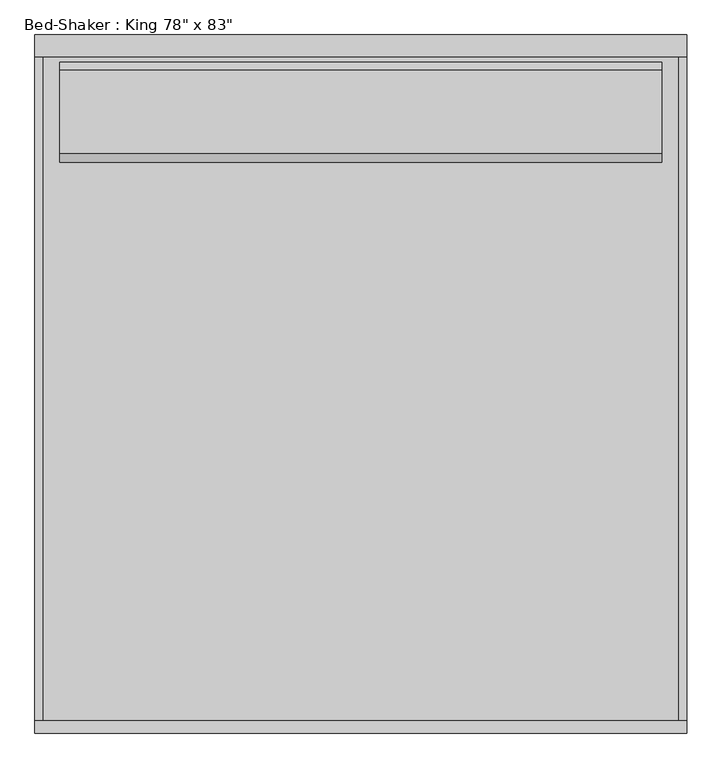
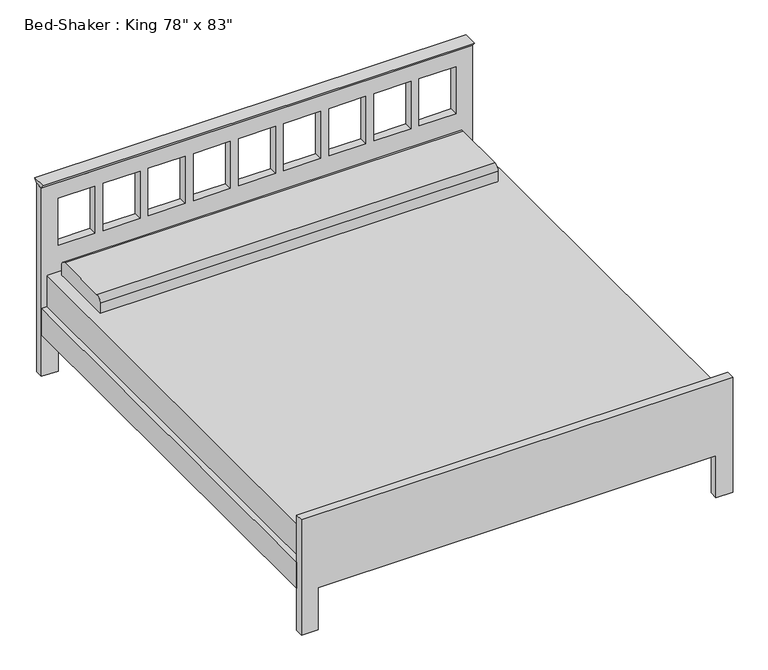
"""IFC4 building model written with IfcOpenShell, lengths in millimetres: furniture geometry."""

from ifc_helpers import new_model, si_unit, point, frame, frame_2d, origin, place, context, project, spatial, polyline, circle_curve, trimmed, segment, composite_curve, outline, extrude, source, transform, mapped, element, save


def furniture_b8e5f23d(model_context):
    return source(origin(), model_context, "Body", "SweptSolid", [
        extrude(outline(polyline([(914.4, 971.8168067), (914.4, -1009.4365546), (0.0, -1009.4365546), (0.0, -933.45), (203.2, -933.45), (203.2, 895.35), (0.0, 895.35), (0.0, 971.8168067), (914.4, 971.8168067)]), holes=[polyline([(838.2, -764.1166667), (609.6, -764.1166667), (609.6, -933.45), (838.2, -933.45), (838.2, -764.1166667)]), polyline([(838.2, -556.6833333), (609.6, -556.6833333), (609.6, -726.0166667), (838.2, -726.0166667), (838.2, -556.6833333)]), polyline([(838.2, -349.25), (609.6, -349.25), (609.6, -518.5833333), (838.2, -518.5833333), (838.2, -349.25)]), polyline([(838.2, -141.8166667), (609.6, -141.8166667), (609.6, -311.15), (838.2, -311.15), (838.2, -141.8166667)]), polyline([(838.2, 273.05), (609.6, 273.05), (609.6, 103.7166667), (838.2, 103.7166667), (838.2, 273.05)]), polyline([(838.2, 480.4833333), (609.6, 480.4833333), (609.6, 311.15), (838.2, 311.15), (838.2, 480.4833333)]), polyline([(838.2, 687.9166667), (609.6, 687.9166667), (609.6, 518.5833333), (838.2, 518.5833333), (838.2, 687.9166667)]), polyline([(838.2, 895.35), (609.6, 895.35), (609.6, 726.0166667), (838.2, 726.0166667), (838.2, 895.35)]), polyline([(838.2, 65.6166667), (609.6, 65.6166667), (609.6, -103.7166667), (838.2, -103.7166667), (838.2, 65.6166667)])]), frame((0.0, -38.1, 0.0), z_axis=(0.0, 1.0, 0.0), x_axis=(0.0, 0.0, 1.0)), (0.0, 0.0, 1.0), 38.1),
        extrude(outline(polyline([(0.0, -933.45), (203.2, -933.45), (203.2, 895.35), (0.0, 895.35), (0.0, 971.55), (558.8, 971.55), (558.8, -1009.65), (0.0, -1009.65), (0.0, -933.45)])), frame((0.0, -2108.2, 0.0), z_axis=(0.0, 1.0, 0.0), x_axis=(0.0, 0.0, 1.0)), (0.0, 0.0, 1.0), 38.1),
        extrude(outline(polyline([(-1009.65, -2070.1), (-1009.65, -38.1), (-984.25, -38.1), (-984.25, -2070.1), (-1009.65, -2070.1)])), frame((0.0, 0.0, 203.5755296), z_axis=(0.0, 0.0, 1.0), x_axis=(1.0, 0.0, 0.0)), (0.0, 0.0, 1.0), 127.0),
        extrude(outline(polyline([(946.15, -2070.1), (946.15, -38.1), (971.55, -38.1), (971.55, -2070.1), (946.15, -2070.1)])), frame((0.0, 0.0, 203.0994861), z_axis=(0.0, 0.0, 1.0), x_axis=(1.0, 0.0, 0.0)), (0.0, 0.0, 1.0), 127.0),
        extrude(outline(polyline([(946.15, -38.1), (946.15, -2070.1), (-984.25, -2070.1), (-984.25, -38.1), (946.15, -38.1)])), frame((0.0, 0.0, 228.6), z_axis=(0.0, 0.0, 1.0), x_axis=(1.0, 0.0, 0.0)), (0.0, 0.0, 1.0), 254.0),
        extrude(outline(composite_curve([segment(polyline([(-373.2486637, 482.6), (-373.2486637, 533.4)]), True, "CONTINUOUS"), segment(trimmed(circle_curve(frame_2d((-347.8486637, 533.4)), 25.4), [point((-373.2486637, 533.4))], [point((-347.8486637, 558.8))], False, "CARTESIAN"), True, "CONTINUOUS"), segment(polyline([(-347.8486637, 558.8), (-93.8486637, 558.8)]), True, "CONTINUOUS"), segment(trimmed(circle_curve(frame_2d((-93.8486637, 533.4)), 25.4), [point((-93.8486637, 558.8))], [point((-68.4486637, 533.4))], False, "CARTESIAN"), True, "CONTINUOUS"), segment(polyline([(-68.4486637, 533.4), (-68.4486637, 482.6), (-373.2486637, 482.6)]), True, "CONTINUOUS")], self_intersect=False)), frame((-933.45, 0.0, 0.0), z_axis=(1.0, 0.0, 0.0), x_axis=(0.0, 1.0, 0.0)), (0.0, 0.0, 1.0), 1828.8),
        extrude(outline(polyline([(-38.1, 914.4), (-51.9545455, 933.45), (13.8545455, 933.45), (0.0, 914.4), (-38.1, 914.4)])), frame((-1009.4365546, 0.0, 0.0), z_axis=(1.0, 0.0, 0.0), x_axis=(0.0, 1.0, 0.0)), (0.0, 0.0, 1.0), 1981.2533613),
    ])


if __name__ == "__main__":
    model = new_model("IFC4")
    model_context = context("Model", 3, world=origin())
    ifc_project = project(units=[si_unit("LENGTHUNIT", "METRE", prefix="MILLI")], contexts=[model_context])
    site = spatial("IfcSite", under=ifc_project)
    building = spatial("IfcBuilding", under=site)
    placement = place(None, origin())
    furniture_shape = furniture_b8e5f23d(model_context)
    element("IfcFurniture", 1, ObjectType="Bed-Shaker : King 78\" x 83\"", at=placement, inside=building, context=model_context, shape_type="MappedRepresentation", body=[
        mapped(furniture_shape, transform((0.0, 0.0, 0.0), x_axis=(1.0, 0.0, 0.0), y_axis=(0.0, 1.0, 0.0), z_axis=(0.0, 0.0, 1.0))),
    ])
    save(model, "model.ifc")

# Revit data of these elements
# Type "Bed-Shaker : King 78\" x 83\""
#   Assembly Code = "E2020200"
#   Length = 2108.2 mm
#   Width = 1981.2 mm
#   Frame Material = Birch
#   Mattress Material = Linen, White
#   Default Elevation = 0
# Element 1 (IfcFurniture, "Bed-Shaker : King 78\" x 83\"")
#   Materials on its faces: "Birch", "Linen, White"
# Materials
#   "Birch": class "Wood", colour RGB 224 178 126, transparency 0, Description = "Betula Alleghaniensis", Cost = 0
#   "Linen, White": class "Textile", colour RGB 247 247 239, transparency 0, Description = "Linen, white", Cost = 0
